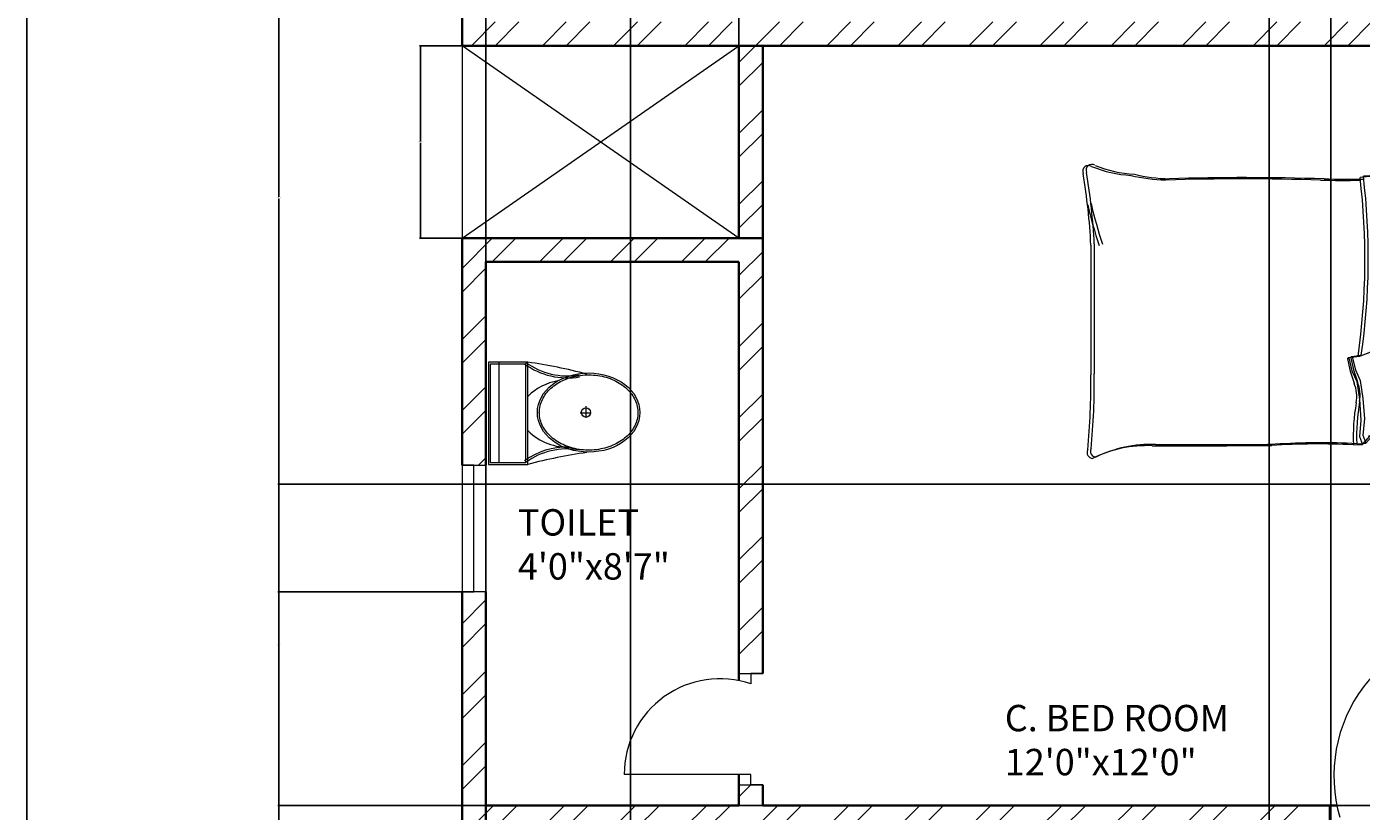
# Model space of a CAD drawing. Units: inches. Extents: x 1965 to 2673, y 1802 to 2669.
# Tile 7 of 16: x 1965 to 2218, y 2267 to 2416. Entities that reach past the tile are written whole.
import ezdxf

# ---------------------------------------------------------------- set-up
doc = ezdxf.new("R2010")
doc.units = ezdxf.units.IN
for name, color, linetype, lineweight in [('A-ANNO-DIMS', 2, 'Continuous', 18), ('A-ANNO-TTLB', 7, 'Continuous', 25), ('A-AREA-IDEN', 7, 'Continuous', 18), ('A-DOOR', 11, 'Continuous', 18), ('A-FLOR-FIXT', 9, 'Continuous', 18), ('A-FLOR-OPEN', 8, 'Continuous', 13), ('A-FURN', 8, 'Continuous', 13), ('A-GLAZ', 181, 'Continuous', 18), ('A-WALL', 7, 'Continuous', 35), ('A-WALL-PATT', 252, 'Continuous', 13)]:
    doc.layers.add(name, color=color, linetype=linetype, lineweight=lineweight)
doc.styles.get("Standard").update_dxf_attribs({"font": 'arial.ttf'})
doc.dimstyles.get("Standard").update_dxf_attribs({"dimtxt": 0.18, "dimasz": 0.18, "dimexe": 0.18, "dimexo": 0.0625, "dimgap": 0.09, "dimtad": 0, "dimtih": 1, "dimtoh": 1, "dimdec": 4, "dimzin": 0, "dimdsep": 46, "dimtxsty": 'Standard', "dimcen": 0.09, "dimadec": 0, "dimazin": 0, "dimtfac": 1, "dimtdec": 4, "dimtofl": 0, "dimtmove": 0, "dimatfit": 3, "dimfxl": 1, "dimtolj": 1, "dimtzin": 0, "dimarcsym": 0})

# ---------------------------------------------------------------- blocks, each defined once
blk = doc.blocks.new('A$C31115884')
for p, q in [((283.1, 497.7), (223.4, 497.7)), ((257.5, 466.4), (257.5, 523.2)), ((0, 200), (0, 0)), ((520, 200), (0, 200)), ((10, 190), (10, 10)), ((510, 190), (10, 190)), ((510, 10), (510, 190)), ((520, 0), (520, 200)), ((510, 54.5), (0, 54.5)), ((10, 10), (510, 10)), ((0, 0), (520, 0))]:
    blk.add_line(p, q)
blk.add_circle((255.6, 496.4), 23.6)
for centre, radius, start, end in [((2777.7, -204.6), 2807, 165.4549, 171.71327), ((3237, 905), 2807, 188.28673, 194.5451), ((-294.5, 403.3), 364.7, 324.20913, 9.34987), ((-294.5, 403.3), 374.7, 324.20913, 9.34987), ((139.5, 406.2), 293.5, 315.84364, 2.65635), ((805.8, 403.3), 374.7, 179.20365, 215.79087), ((805.8, 403.3), 364.7, 170.65013, 215.79087), ((383.6, 406.2), 293.5, 190.27735, 224.15636)]:
    blk.add_arc(centre, radius, start, end)
blk.add_ellipse((256.2, 509.9), major_axis=(0, -260.7), ratio=0.772727)
blk.add_open_spline([(256.2, 259.2), (263.1, 259.2), (270, 259.7), (287.8, 262.3), (298.7, 265.1), (319.9, 273.1), (330.2, 278.4), (350.1, 291.1), (359.7, 298.7), (377.7, 315.9), (386.2, 325.5), (401.7, 346.6), (408.8, 358.1), (421.3, 382.5), (426.8, 395.5), (435.9, 422.4), (439.5, 436.4), (444.8, 465.1), (446.5, 479.7), (447.9, 509.2), (447.6, 524), (445, 553.3), (442.7, 567.8), (436.3, 596), (432.1, 609.7), (421.9, 636), (416, 648.6), (402.5, 672.1), (395, 683), (378.6, 703), (369.8, 712.1), (351.1, 728), (341.3, 734.8), (320.9, 746.2), (310.4, 750.7), (288.9, 757.3), (278, 759.4), (256, 761), (245, 760.6), (223.1, 757.2), (212.3, 754.3), (191.1, 746.1), (180.8, 740.7), (160.9, 727.8), (151.4, 720.1), (133.5, 702.7), (125.1, 693), (109.6, 671.7), (102.6, 660.2), (90.2, 635.7), (84.9, 622.7), (76, 595.6), (72.4, 581.6), (67.2, 552.9), (65.6, 538.2), (64.4, 508.8), (64.8, 494), (67.5, 464.7), (69.9, 450.2), (76.6, 422), (80.8, 408.3), (91.1, 382.2), (97.2, 369.7), (110.8, 346.3), (118.4, 335.4), (134.8, 315.6), (143.7, 306.7), (162.4, 290.9), (172.3, 284.2), (192.8, 273), (203.3, 268.6), (224.8, 262.2), (235.8, 260.2), (249.9, 259.3), (253, 259.2), (256.2, 259.2)], degree=3, knots=[0, 0, 0, 0, 0.110105, 0.110105, 0.285049, 0.285049, 0.459994, 0.459994, 0.634938, 0.634938, 0.809882, 0.809882, 0.984827, 0.984827, 1.159771, 1.159771, 1.334715, 1.334715, 1.50966, 1.50966, 1.684604, 1.684604, 1.859549, 1.859549, 2.034493, 2.034493, 2.209437, 2.209437, 2.384382, 2.384382, 2.559326, 2.559326, 2.73427, 2.73427, 2.909215, 2.909215, 3.084159, 3.084159, 3.259103, 3.259103, 3.434048, 3.434048, 3.608992, 3.608992, 3.783936, 3.783936, 3.958881, 3.958881, 4.133825, 4.133825, 4.30877, 4.30877, 4.483714, 4.483714, 4.658658, 4.658658, 4.833603, 4.833603, 5.008547, 5.008547, 5.183491, 5.183491, 5.358436, 5.358436, 5.53338, 5.53338, 5.708324, 5.708324, 5.883269, 5.883269, 6.058213, 6.058213, 6.233158, 6.233158, 6.283185, 6.283185, 6.283185, 6.283185])
blk = doc.blocks.new('BED-DOUBLE')
for p, q in [((3.47, 63.33), (3.47, 81.44)), ((3.47, 63.33), (3.47, 81.44)), ((3.47, 81.44), (51.49, 81.44)), ((51.26, 81.44), (51.26, 54.83)), ((51.26, 81.44), (51.26, 54.83)), ((51.49, 81.44), (51.49, 80.8)), ((3.47, 79.91), (51.26, 79.91)), ((3.47, 79.91), (51.26, 79.91)), ((3.7, 62.69), (3.7, 80.8)), ((3.7, 62.69), (3.7, 80.8)), ((3.7, 79.27), (51.49, 79.27)), ((3.7, 79.27), (51.49, 79.27)), ((3.89, 78.1), (8.17, 78.43)), ((3.89, 78.1), (8.17, 78.43)), ((8.17, 78.43), (8.28, 78.41)), ((8.17, 78.43), (8.28, 78.41)), ((16.87, 78.41), (19.76, 79.14)), ((16.87, 78.41), (19.76, 79.14)), ((17.1, 77.77), (19.99, 78.5)), ((17.1, 77.77), (19.99, 78.5)), ((19.76, 79.14), (20.09, 79.14)), ((19.76, 79.14), (20.09, 79.14)), ((19.99, 78.5), (20.31, 78.5)), ((19.99, 78.5), (20.31, 78.5)), ((20.09, 79.14), (24.53, 78.99)), ((20.09, 79.14), (24.53, 78.99)), ((20.31, 78.5), (24.76, 78.35)), ((20.31, 78.5), (24.76, 78.35)), ((24.53, 78.99), (25.98, 79.57)), ((24.53, 78.99), (25.98, 79.57)), ((24.76, 78.35), (26.21, 78.93)), ((24.76, 78.35), (26.21, 78.93)), ((25.98, 79.57), (26.56, 74.22)), ((25.98, 79.57), (26.56, 74.22)), ((26.21, 78.93), (26.78, 73.58)), ((26.21, 78.93), (26.78, 73.58)), ((27.97, 78.95), (27.73, 73.57)), ((27.97, 78.95), (27.73, 73.57)), ((29.45, 78.46), (27.97, 78.95)), ((29.45, 78.46), (27.97, 78.95)), ((33.88, 78.88), (29.45, 78.46)), ((33.88, 78.88), (29.45, 78.46)), ((34.2, 78.9), (33.88, 78.88)), ((34.2, 78.9), (33.88, 78.88)), ((37.13, 78.36), (34.2, 78.9)), ((37.13, 78.36), (34.2, 78.9)), ((45.71, 78.9), (41.91, 78.37)), ((45.71, 78.9), (41.91, 78.37)), ((50.11, 78.88), (44.7, 78.98)), ((44.7, 78.98), (45.71, 78.9)), ((50.11, 78.88), (44.7, 78.98)), ((44.7, 78.98), (45.71, 78.9)), ((50.11, 78.88), (49.73, 75.67)), ((50.11, 78.88), (49.73, 75.67)), ((51.49, 80.8), (51.49, 54.19)), ((51.49, 80.8), (51.49, 54.19)), ((3.89, 78.12), (4.47, 74.94)), ((3.89, 78.12), (4.47, 74.94)), ((4.12, 77.46), (8.4, 77.79)), ((4.12, 77.46), (8.4, 77.79)), ((4.12, 77.49), (4.7, 74.3)), ((4.12, 77.49), (4.7, 74.3)), ((8.28, 78.41), (12.1, 78.12)), ((8.28, 78.41), (12.1, 78.12)), ((8.4, 77.79), (8.51, 77.77)), ((8.4, 77.79), (8.51, 77.77)), ((8.51, 77.77), (12.33, 77.49)), ((8.51, 77.77), (12.33, 77.49)), ((12.1, 78.12), (17.6, 77.11)), ((12.1, 78.12), (17.6, 77.11)), ((12.33, 77.49), (17.82, 76.47)), ((12.33, 77.49), (17.82, 76.47)), ((14.85, 77.69), (16.87, 78.41)), ((14.85, 77.69), (16.87, 78.41)), ((15.08, 77.05), (17.1, 77.77)), ((15.08, 77.05), (17.1, 77.77)), ((28.2, 78.31), (27.96, 72.93)), ((28.2, 78.31), (27.96, 72.93)), ((29.68, 77.82), (28.2, 78.31)), ((29.68, 77.82), (28.2, 78.31)), ((34.11, 78.24), (29.68, 77.82)), ((34.11, 78.24), (29.68, 77.82)), ((34.43, 78.26), (34.11, 78.24)), ((34.43, 78.26), (34.11, 78.24)), ((37.36, 77.72), (34.43, 78.26)), ((37.36, 77.72), (34.43, 78.26)), ((41.91, 78.37), (36.49, 77.02)), ((41.91, 78.37), (36.49, 77.02)), ((42.14, 77.73), (36.72, 76.38)), ((42.14, 77.73), (36.72, 76.38)), ((39.2, 77.77), (37.13, 78.36)), ((39.19, 77.77), (37.13, 78.36)), ((39.42, 77.13), (37.36, 77.72)), ((39.42, 77.13), (37.36, 77.72)), ((45.94, 78.26), (42.14, 77.73)), ((45.94, 78.26), (42.14, 77.73)), ((50.34, 78.24), (44.93, 78.34)), ((44.93, 78.34), (45.94, 78.26)), ((50.34, 78.24), (44.93, 78.34)), ((44.93, 78.34), (45.94, 78.26)), ((50.34, 78.24), (49.96, 75.03)), ((50.34, 78.24), (49.96, 75.03)), ((4.47, 74.94), (4.03, 72.34)), ((4.47, 74.94), (4.03, 72.34)), ((4.7, 74.3), (4.26, 71.7)), ((4.7, 74.3), (4.26, 71.7)), ((5.05, 72.49), (6.06, 75.23)), ((5.05, 72.49), (6.06, 75.23)), ((5.27, 71.85), (6.29, 74.59)), ((5.27, 71.85), (6.29, 74.59)), ((26.56, 74.22), (27.13, 71.04)), ((26.56, 74.22), (27.13, 71.04)), ((26.78, 73.58), (27.36, 70.4)), ((26.78, 73.58), (27.36, 70.4)), ((27.73, 73.57), (27.35, 70.36)), ((27.73, 73.57), (27.35, 70.36)), ((49.3, 73.18), (48.12, 75.86)), ((49.3, 73.18), (48.12, 75.86)), ((49.53, 72.54), (48.35, 75.22)), ((49.53, 72.54), (48.35, 75.22)), ((49.73, 75.67), (50.32, 73.1)), ((49.73, 75.67), (50.32, 73.1)), ((49.96, 75.03), (50.55, 72.46)), ((49.96, 75.03), (50.55, 72.46)), ((4.03, 72.34), (4.61, 71.33)), ((4.03, 72.34), (4.61, 71.33)), ((4.26, 71.7), (4.84, 70.69)), ((4.26, 71.7), (4.84, 70.69)), ((4.47, 68.87), (5.05, 72.49)), ((4.47, 68.87), (5.05, 72.49)), ((4.7, 68.23), (5.27, 71.85)), ((4.7, 68.23), (5.27, 71.85)), ((27.13, 71.04), (27.13, 69.74)), ((27.13, 71.04), (27.13, 69.74)), ((27.96, 72.93), (27.58, 69.72)), ((27.96, 72.93), (27.58, 69.72)), ((50.11, 69.61), (49.3, 73.18)), ((50.11, 69.61), (49.3, 73.18)), ((50.34, 68.97), (49.53, 72.54)), ((50.34, 68.97), (49.53, 72.54)), ((50.32, 73.1), (49.81, 72.06)), ((50.32, 73.1), (49.81, 72.06)), ((50.55, 72.46), (50.04, 71.42)), ((50.55, 72.46), (50.04, 71.42)), ((4.76, 67.28), (4.47, 68.87)), ((4.76, 67.28), (4.47, 68.87)), ((27.13, 69.74), (26.56, 67.86)), ((27.13, 69.74), (26.56, 67.86)), ((27.36, 69.1), (26.78, 67.22)), ((27.36, 69.1), (26.78, 67.22)), ((27.35, 70.36), (27.43, 69.06)), ((27.35, 70.36), (27.43, 69.06)), ((27.36, 70.4), (27.36, 69.1)), ((27.36, 70.4), (27.36, 69.1)), ((27.43, 69.06), (28.13, 67.22)), ((27.43, 69.06), (28.13, 67.22)), ((27.58, 69.72), (27.66, 68.42)), ((27.58, 69.72), (27.66, 68.42)), ((27.66, 68.42), (28.35, 66.58)), ((27.66, 68.42), (28.35, 66.58)), ((49.92, 68.01), (50.11, 69.61)), ((49.92, 68.01), (50.11, 69.61)), ((50.15, 67.37), (50.34, 68.97)), ((50.15, 67.37), (50.34, 68.97)), ((4.18, 64.1), (4.76, 67.28)), ((4.18, 64.1), (4.76, 67.28)), ((4.41, 63.46), (4.99, 66.64)), ((4.41, 63.46), (4.99, 66.64)), ((4.99, 66.64), (4.7, 68.23)), ((4.99, 66.64), (4.7, 68.23)), ((6.38, 65.81), (10.41, 65.15)), ((6.38, 65.81), (10.41, 65.15)), ((24.1, 65.18), (20.95, 66.27)), ((24.1, 65.18), (20.95, 66.27)), ((26.56, 67.86), (26.56, 65.18)), ((26.56, 67.86), (26.56, 65.18)), ((26.78, 67.22), (26.78, 64.54)), ((26.78, 67.22), (26.78, 64.54)), ((28.13, 67.22), (28.29, 64.55)), ((28.13, 67.22), (28.29, 64.55)), ((28.35, 66.58), (28.52, 63.91)), ((28.35, 66.58), (28.52, 63.91)), ((30.75, 64.7), (33.82, 65.99)), ((30.75, 64.7), (33.82, 65.99)), ((32.56, 65.81), (36.59, 65.15)), ((32.56, 65.81), (36.59, 65.15)), ((50.69, 64.87), (49.92, 68.01)), ((50.69, 64.87), (49.92, 68.01)), ((50.92, 64.23), (50.15, 67.37)), ((50.92, 64.23), (50.15, 67.37)), ((9.28, 64.82), (4.18, 64.1)), ((9.28, 64.82), (4.18, 64.1)), ((9.5, 64.18), (4.41, 63.46)), ((9.5, 64.18), (4.41, 63.46)), ((6.6, 65.17), (10.64, 64.51)), ((6.61, 65.17), (10.64, 64.51)), ((10.41, 65.15), (9.28, 64.82)), ((10.41, 65.15), (9.28, 64.82)), ((10.64, 64.51), (9.5, 64.18)), ((10.64, 64.51), (9.5, 64.18)), ((10.41, 65.15), (17.42, 64.71)), ((10.41, 65.15), (17.42, 64.71)), ((10.64, 64.51), (17.65, 64.08)), ((10.64, 64.51), (17.65, 64.08)), ((17.42, 64.71), (19.38, 65.27)), ((17.42, 64.71), (19.38, 65.27)), ((17.65, 64.08), (19.61, 64.63)), ((17.65, 64.08), (19.61, 64.63)), ((19.38, 65.27), (24.51, 64.87)), ((19.38, 65.27), (24.51, 64.87)), ((19.61, 64.63), (24.74, 64.23)), ((19.61, 64.63), (24.74, 64.23)), ((24.33, 64.54), (21.18, 65.63)), ((24.33, 64.54), (21.18, 65.63)), ((26.56, 65.18), (24.1, 65.18)), ((26.56, 65.18), (24.1, 65.18)), ((26.78, 64.54), (24.33, 64.54)), ((26.78, 64.54), (24.33, 64.54)), ((28.29, 64.55), (30.75, 64.7)), ((28.29, 64.55), (30.75, 64.7)), ((28.52, 63.91), (30.97, 64.06)), ((28.52, 63.91), (30.97, 64.06)), ((30.25, 64.06), (34.44, 57.56)), ((30.25, 64.06), (34.44, 57.56)), ((30.48, 63.42), (34.67, 56.92)), ((30.48, 63.42), (34.67, 56.92)), ((30.97, 64.06), (34.04, 65.35)), ((30.97, 64.06), (34.04, 65.35)), ((40.64, 61.12), (32.3, 64.06)), ((40.64, 61.12), (32.3, 64.06)), ((40.87, 60.48), (32.53, 63.42)), ((40.87, 60.48), (32.53, 63.42)), ((32.79, 65.17), (36.82, 64.51)), ((32.79, 65.17), (36.82, 64.51)), ((36.59, 65.15), (43.6, 64.71)), ((36.59, 65.15), (43.6, 64.71)), ((36.82, 64.51), (43.83, 64.08)), ((36.82, 64.51), (43.83, 64.08)), ((43.6, 64.71), (45.56, 65.27)), ((43.6, 64.71), (45.56, 65.27)), ((43.83, 64.08), (45.79, 64.63)), ((43.83, 64.08), (45.79, 64.63)), ((45.56, 65.27), (50.69, 64.87)), ((45.56, 65.27), (50.69, 64.87)), ((45.79, 64.63), (50.92, 64.23)), ((45.79, 64.63), (50.92, 64.23)), ((46.21, 59.11), (40.64, 61.12)), ((46.21, 59.11), (40.64, 61.12)), ((46.44, 58.47), (40.87, 60.48)), ((46.44, 58.47), (40.87, 60.48)), ((49.16, 56.95), (46.21, 59.11)), ((49.16, 56.95), (46.21, 59.11)), ((49.39, 56.31), (46.44, 58.47)), ((49.39, 56.31), (46.44, 58.47)), ((34.44, 57.56), (36.15, 53.08)), ((34.44, 57.56), (36.15, 53.08)), ((34.67, 56.92), (36.38, 52.44)), ((34.67, 56.92), (36.38, 52.44)), ((52.86, 53.69), (49.16, 56.95)), ((52.86, 53.69), (49.16, 56.95)), ((53.09, 53.06), (49.39, 56.31)), ((53.09, 53.06), (49.39, 56.31)), ((44.36, 53.08), (48.23, 53.39)), ((44.36, 53.08), (48.23, 53.39)), ((48.23, 53.39), (51.33, 53.08)), ((48.23, 53.39), (51.33, 53.08)), ((51.33, 53.08), (52.86, 53.69)), ((51.33, 53.08), (52.86, 53.69)), ((52.94, 51.95), (52.86, 53.69, 3.87)), ((52.94, 51.95), (52.86, 53.69, 3.87)), ((36.15, 53.08), (36.46, 51.06)), ((36.15, 53.08), (36.46, 51.06)), ((36.38, 52.44), (36.69, 50.42)), ((36.38, 52.44), (36.69, 50.42)), ((36.46, 51.06), (38.94, 51.68)), ((36.46, 51.06), (38.94, 51.68)), ((36.69, 50.42), (39.16, 51.04)), ((36.69, 50.42), (39.16, 51.04)), ((38.94, 51.68), (40.95, 52.61)), ((38.94, 51.68), (40.95, 52.61)), ((39.16, 51.04), (41.18, 51.97)), ((39.16, 51.04), (41.18, 51.97)), ((40.95, 52.61), (44.36, 53.08)), ((40.95, 52.61), (44.36, 53.08)), ((41.18, 51.97), (44.58, 52.44)), ((41.18, 51.97), (44.58, 52.44)), ((44.58, 52.44), (48.46, 52.75)), ((44.58, 52.44), (48.46, 52.75)), ((48.46, 52.75), (51.55, 52.44)), ((48.46, 52.75), (51.55, 52.44)), ((51.55, 52.44), (53.09, 53.06)), ((51.55, 52.44), (53.09, 53.06)), ((53.17, 51.31), (53.09, 53.06, 3.87)), ((53.17, 51.31), (53.09, 53.06, 3.87)), ((15.06, 2.2), (39.67, 2.2)), ((15.06, 2.2), (39.67, 2.2)), ((15.29, 1.56), (39.9, 1.56)), ((15.29, 1.56), (39.9, 1.56))]:
    blk.add_line(p, q)
for centre, radius, start, end in [((21.35, -100.61), 164.97, 86.0865, 96.7821), ((21.35, -100.61), 164.97, 86.0865, 96.7821), ((21.58, -101.25), 164.97, 86.0865, 96.7821), ((21.58, -101.25), 164.97, 86.0865, 96.7821), ((85.16, 61.34), 83.31, 178.7218, 185.604), ((85.16, 61.34), 83.31, 178.7218, 185.604), ((85.39, 60.71), 83.31, 178.7218, 185.604), ((85.38, 60.71), 83.31, 178.7218, 185.604), ((17.75, -74.88), 129.02, 81.7845, 96.9006), ((17.75, -74.88), 129.02, 81.7845, 96.9006), ((17.98, -75.51), 129.02, 81.7845, 96.9006), ((17.98, -75.51), 129.02, 81.7845, 96.9006), ((-167.31, 50.27), 170.11, 358.4762, 1.0082), ((-167.31, 50.27), 170.11, 358.4762, 1.0082), ((-167.08, 49.63), 170.11, 358.4762, 1.0082), ((-167.08, 49.63), 170.11, 358.4762, 1.0082), ((36.63, 51), 0.185, 160.2464, 271.1377), ((36.63, 51), 0.185, 160.2464, 271.1377), ((31.15, 79.96), 29.65, 280.6617, 289.8806), ((31.15, 79.96), 29.65, 280.6617, 289.8806), ((31.38, 79.32), 29.65, 280.6617, 289.8806), ((31.38, 79.32), 29.65, 280.6617, 289.8806), ((43.74, 46.37), 6.22, 78.6608, 113.7384), ((43.74, 46.37), 6.22, 78.6608, 113.7384), ((43.97, 45.74), 6.22, 78.6608, 113.7384), ((43.97, 45.74), 6.22, 78.6608, 113.7384), ((51.32, 88.1), 36.18, 259.8763, 272.5657), ((51.32, 88.1), 36.18, 259.8763, 272.5657), ((51.55, 87.46), 36.18, 259.8763, 272.5657), ((51.55, 87.46), 36.18, 259.8763, 272.5657), ((182.26, 45.13), 129.5, 176.9791, 183.8365), ((182.26, 45.13), 129.5, 176.9791, 183.8365), ((182.49, 44.49), 129.5, 176.9791, 183.8365), ((182.49, 44.49), 129.5, 176.9791, 183.8365), ((36.86, 50.36), 0.185, 160.2464, 271.1377), ((36.86, 50.36), 0.185, 160.2464, 271.1377), ((484.82, 30.83), 482.31, 178.2277, 181.7185), ((484.82, 30.83), 482.31, 178.2277, 181.7185), ((485.05, 30.19), 482.31, 178.2277, 181.7185), ((485.05, 30.19), 482.31, 178.2277, 181.7185), ((-4508.75, 13.62), 4561.86, 0.00217, 0.28689), ((-4508.75, 13.62), 4561.86, 0.00217, 0.28689), ((-4508.52, 12.98), 4561.86, 0.00217, 0.28689), ((-4508.52, 12.98), 4561.86, 0.00217, 0.28689), ((-26.9, 16.93), 29.63, 346.0648, 358.9113), ((-26.9, 16.93), 29.63, 346.0648, 358.9113), ((-26.68, 16.29), 29.63, 346.0648, 358.9113), ((-26.68, 16.29), 29.63, 346.0648, 358.9113), ((76.15, 12.77), 23.07, 177.4714, 206.4681), ((76.15, 12.77), 23.07, 177.4714, 206.4681), ((76.38, 12.14), 23.07, 177.4714, 206.4681), ((76.38, 12.14), 23.07, 177.4714, 206.4681), ((-21.66, 11.17), 23.56, 337.9751, 356.652), ((-21.66, 11.17), 23.56, 337.9751, 356.652), ((-21.44, 10.53), 23.56, 337.9751, 356.652), ((-21.44, 10.53), 23.56, 337.9751, 356.652), ((-17.23, 105.15), 106.46, 283.3832, 287.7053), ((-17.23, 105.15), 106.46, 283.3832, 287.7053), ((-17, 104.51), 106.46, 283.3832, 287.7053), ((-17, 104.51), 106.46, 283.3832, 287.7053), ((1.08, 1.72), 1.09, 146.1736, 293.4781), ((1.08, 1.72), 1.09, 146.1736, 293.4781), ((1.31, 1.08), 1.09, 146.1736, 293.4781), ((1.31, 1.08), 1.09, 146.1736, 293.4781), ((21.42, -119.4), 121.76, 92.9958, 99.4091), ((21.42, -119.4), 121.76, 92.9958, 99.4091), ((21.65, -120.04), 121.76, 92.9958, 99.4091), ((21.65, -120.04), 121.76, 92.9958, 99.4091), ((41.15, -130.84), 133.04, 84.4998, 90.6351), ((41.15, -130.84), 133.04, 84.4998, 90.6351), ((41.38, -131.48), 133.04, 84.4998, 90.6351), ((41.37, -131.48), 133.04, 84.4998, 90.6351), ((54.4, 2.57), 1.1, 242.6588, 356.02), ((54.4, 2.57), 1.1, 242.6588, 356.02), ((54.63, 1.93), 1.1, 242.6588, 356.02), ((54.63, 1.93), 1.1, 242.6588, 356.02)]:
    blk.add_arc(centre, radius, start, end)
blk = doc.blocks.new('SHAFT-OPENING')
for p, q in [((0, 36.5), (0, 0)), ((52.5, 0), (0, 36.5)), ((0, 0), (52.5, 36.5))]:
    blk.add_line(p, q)
blk = doc.blocks.new('*D23')
at = {"layer": 'A-ANNO-DIMS', "color": 0, "lineweight": -2, "transparency": 16777216}
for p, q in [((2047.09, 2412.65), (2047.09, 2420.65)), ((2047.27, 2420.47), (2072.37, 2420.47)), ((2099.41, 2420.47), (2074.32, 2420.47)), ((2099.59, 2412.65), (2099.59, 2420.65))]:
    blk.add_line(p, q, dxfattribs=at)
at = {"layer": 'A-ANNO-DIMS', "color": 0, "transparency": 16777216}
for points in [[(2047.27, 2420.5), (2047.27, 2420.44), (2047.09, 2420.47)], [(2099.41, 2420.5), (2099.41, 2420.44), (2099.59, 2420.47)]]:
    blk.add_solid(points, dxfattribs=at)
at = {"layer": 'Defpoints', "color": 0, "transparency": 16777216}
for p in [(2099.59, 2420.47), (2047.09, 2412.59), (2099.59, 2412.59)]:
    blk.add_point(p, dxfattribs=at)
at = {"layer": 'A-ANNO-DIMS', "color": 0, "transparency": 16777216, "insert": (2073.34, 2420.47), "char_height": 0.18, "attachment_point": 5}
blk.add_mtext('\\A1;SHAFT 53 TYP.', dxfattribs=at)
blk = doc.blocks.new('*D24')
at = {"layer": 'A-ANNO-DIMS', "color": 0, "lineweight": -2, "transparency": 16777216}
for p, q in [((2047.03, 2412.59), (2039.04, 2412.59)), ((2039.22, 2412.41), (2039.22, 2394.52)), ((2039.22, 2376.27), (2039.22, 2394.16)), ((2047.03, 2376.09), (2039.04, 2376.09))]:
    blk.add_line(p, q, dxfattribs=at)
at = {"layer": 'A-ANNO-DIMS', "color": 0, "transparency": 16777216}
for points in [[(2039.19, 2412.41), (2039.25, 2412.41), (2039.22, 2412.59)], [(2039.19, 2376.27), (2039.25, 2376.27), (2039.22, 2376.09)]]:
    blk.add_solid(points, dxfattribs=at)
at = {"layer": 'Defpoints', "color": 0, "transparency": 16777216}
for p in [(2039.22, 2412.59), (2047.09, 2412.59), (2047.09, 2376.09)]:
    blk.add_point(p, dxfattribs=at)
at = {"layer": 'A-ANNO-DIMS', "color": 0, "transparency": 16777216, "insert": (2039.22, 2394.34), "char_height": 0.18, "attachment_point": 5}
blk.add_mtext('\\A1;37 TYP.', dxfattribs=at)
blk = doc.blocks.new('*D36')
at = {"layer": 'A-ANNO-DIMS', "color": 0, "lineweight": -2, "transparency": 16777216}
for p, q in [((2047.03, 2309.07), (2012.19, 2309.07)), ((2012.37, 2308.89), (2012.37, 2253.51)), ((2012.37, 2197.76), (2012.37, 2253.14)), ((2047.03, 2197.58), (2012.19, 2197.58))]:
    blk.add_line(p, q, dxfattribs=at)
at = {"layer": 'A-ANNO-DIMS', "color": 0, "transparency": 16777216}
for points in [[(2012.34, 2308.89), (2012.4, 2308.89), (2012.37, 2309.07)], [(2012.34, 2197.76), (2012.4, 2197.76), (2012.37, 2197.58)]]:
    blk.add_solid(points, dxfattribs=at)
at = {"layer": 'Defpoints', "color": 0, "transparency": 16777216}
for p in [(2012.37, 2309.07), (2047.09, 2309.07), (2047.09, 2197.58)]:
    blk.add_point(p, dxfattribs=at)
at = {"layer": 'A-ANNO-DIMS', "color": 0, "transparency": 16777216, "insert": (2012.37, 2253.33), "char_height": 0.18, "attachment_point": 5}
blk.add_mtext('\\A1;111.49', dxfattribs=at)
blk = doc.blocks.new('*D37')
at = {"layer": 'A-ANNO-DIMS', "color": 0, "lineweight": -2, "transparency": 16777216}
for p, q in [((2047.03, 2458.38), (2012.19, 2458.38)), ((2012.37, 2458.2), (2012.37, 2383.91)), ((2012.37, 2309.25), (2012.37, 2383.54)), ((2047.03, 2309.07), (2012.19, 2309.07))]:
    blk.add_line(p, q, dxfattribs=at)
at = {"layer": 'A-ANNO-DIMS', "color": 0, "transparency": 16777216}
for points in [[(2012.34, 2458.2), (2012.4, 2458.2), (2012.37, 2458.38)], [(2012.34, 2309.25), (2012.4, 2309.25), (2012.37, 2309.07)]]:
    blk.add_solid(points, dxfattribs=at)
at = {"layer": 'Defpoints', "color": 0, "transparency": 16777216}
for p in [(2012.37, 2458.38), (2047.09, 2458.38), (2047.09, 2309.07)]:
    blk.add_point(p, dxfattribs=at)
at = {"layer": 'A-ANNO-DIMS', "color": 0, "transparency": 16777216, "insert": (2012.37, 2383.73), "char_height": 0.18, "attachment_point": 5}
blk.add_mtext('\\A1;149.3', dxfattribs=at)
blk = doc.blocks.new('*D39')
at = {"layer": 'A-ANNO-DIMS', "color": 0, "lineweight": -2, "transparency": 16777216}
for p, q in [((2051.59, 1936.15), (2051.59, 2600.5)), ((2051.77, 2600.32), (2064.93, 2600.32)), ((2078.87, 2600.32), (2065.72, 2600.32)), ((2079.05, 1936.15), (2079.05, 2600.5))]:
    blk.add_line(p, q, dxfattribs=at)
at = {"layer": 'A-ANNO-DIMS', "color": 0, "transparency": 16777216}
for points in [[(2051.77, 2600.35), (2051.77, 2600.29), (2051.59, 2600.32)], [(2078.87, 2600.35), (2078.87, 2600.29), (2079.05, 2600.32)]]:
    blk.add_solid(points, dxfattribs=at)
at = {"layer": 'Defpoints', "color": 0, "transparency": 16777216}
for p in [(2079.05, 2600.32), (2051.59, 1936.09), (2079.05, 1936.09)]:
    blk.add_point(p, dxfattribs=at)
at = {"layer": 'A-ANNO-DIMS', "color": 0, "transparency": 16777216, "insert": (2065.32, 2600.32), "char_height": 0.18, "attachment_point": 5}
blk.add_mtext('\\A1;27.46', dxfattribs=at)
blk = doc.blocks.new('*D40')
at = {"layer": 'A-ANNO-DIMS', "color": 0, "lineweight": -2, "transparency": 16777216}
for p, q in [((2200.09, 1936.15), (2200.09, 2600.5)), ((2200.27, 2600.32), (2205.48, 2600.32)), ((2211.59, 2600.32), (2206.38, 2600.32)), ((2211.77, 1936.15), (2211.77, 2600.5))]:
    blk.add_line(p, q, dxfattribs=at)
at = {"layer": 'A-ANNO-DIMS', "color": 0, "transparency": 16777216}
for points in [[(2200.27, 2600.35), (2200.27, 2600.29), (2200.09, 2600.32)], [(2211.59, 2600.35), (2211.59, 2600.29), (2211.77, 2600.32)]]:
    blk.add_solid(points, dxfattribs=at)
at = {"layer": 'Defpoints', "color": 0, "transparency": 16777216}
for p in [(2211.77, 2600.32), (2200.09, 1936.09), (2211.77, 1936.09)]:
    blk.add_point(p, dxfattribs=at)
at = {"layer": 'A-ANNO-DIMS', "color": 0, "transparency": 16777216, "insert": (2205.93, 2600.32), "char_height": 0.18, "attachment_point": 5}
blk.add_mtext('\\A1;11.674', dxfattribs=at)
blk = doc.blocks.new('*D48')
at = {"layer": 'A-ANNO-DIMS', "color": 0, "lineweight": -2, "transparency": 16777216}
for p, q in [((2573.53, 2329.47), (2012.19, 2329.47)), ((2012.37, 2329.29), (2012.37, 2299.21)), ((2012.37, 2268.77), (2012.37, 2298.85)), ((2573.53, 2268.59), (2012.19, 2268.59))]:
    blk.add_line(p, q, dxfattribs=at)
at = {"layer": 'A-ANNO-DIMS', "color": 0, "transparency": 16777216}
for points in [[(2012.34, 2329.29), (2012.4, 2329.29), (2012.37, 2329.47)], [(2012.34, 2268.77), (2012.4, 2268.77), (2012.37, 2268.59)]]:
    blk.add_solid(points, dxfattribs=at)
at = {"layer": 'Defpoints', "color": 0, "transparency": 16777216}
for p in [(2012.37, 2329.47), (2573.59, 2329.47), (2573.59, 2268.59)]:
    blk.add_point(p, dxfattribs=at)
at = {"layer": 'A-ANNO-DIMS', "color": 0, "transparency": 16777216, "insert": (2012.37, 2299.03), "char_height": 0.18, "attachment_point": 5}
blk.add_mtext('\\A1;60.87', dxfattribs=at)

msp = doc.modelspace()

# ---------------------------------------------------------------- hatches: boundary and pattern name
at = {"layer": 'A-WALL-PATT'}
h = msp.add_hatch(dxfattribs=at)
h.set_pattern_fill('ANSI32', color=256)
h.paths.add_polyline_path([(2051.5927, 2561.0914), (2076.7559, 2561.0914), (2076.7559, 2563.3414), (2076.7559, 2565.5914), (2047.0927, 2565.5914), (2047.0927, 2518.3824), (2051.5927, 2518.3824)])
h.paths.add_polyline_path([(2051.5927, 2458.3824), (2049.3427, 2458.3824), (2047.0927, 2458.3824), (2047.0927, 2412.5914), (2248.0927, 2412.5914), (2248.0927, 2268.5914), (2252.5927, 2268.5914), (2252.5927, 2412.5914), (2252.5927, 2421.0404), (2250.3427, 2421.0404), (2248.0927, 2421.0404), (2248.0927, 2417.0914), (2051.5927, 2417.0914)])
h.paths.add_polyline_path([(2211.4933, 2268.5914), (2104.0927, 2268.5914), (2104.0927, 2272.4654), (2101.8427, 2272.4654), (2099.5927, 2272.4654), (2099.5927, 2268.5914), (2051.5927, 2268.5914), (2051.5927, 2264.0914), (2147.5927, 2264.0914), (2147.5927, 2259.8893), (2152.0927, 2259.8893), (2152.0927, 2264.0914), (2211.4933, 2264.0914), (2211.4933, 2266.3414)])
h.paths.add_polyline_path([(2104.0927, 2376.0914), (2099.5927, 2376.0914), (2047.0927, 2376.0914), (2047.0927, 2333.0682), (2051.5927, 2333.0682), (2051.5927, 2371.5914), (2099.5927, 2371.5914), (2099.5927, 2293.6123), (2104.0927, 2293.6123)], flags=17)
h.paths.add_polyline_path([(2051.5927, 2309.0682), (2047.0927, 2309.0682), (2047.0927, 2233.5821), (2051.5927, 2233.5821)])
h.paths.add_polyline_path([(2104.0927, 2412.5914), (2099.5927, 2412.5914), (2099.5927, 2376.0914), (2104.0927, 2376.0914)], flags=17)
h.paths.add_polyline_path([(2290.1254, 2268.5914), (2242.4924, 2268.5914), (2242.4924, 2264.0914), (2290.1254, 2264.0914), (2290.1254, 2266.3414)])
h.paths.add_polyline_path([(2284.653, 2264.0914), (2280.153, 2264.0914), (2280.153, 2161.6826), (2284.653, 2161.6826)])
h.paths.add_polyline_path([(2578.0927, 2329.4656), (2573.5927, 2329.4656), (2573.5927, 2268.5914), (2525.5927, 2268.5914), (2525.5927, 2271.9222), (2523.3427, 2271.9222), (2521.0927, 2271.9222), (2521.0927, 2268.5914), (2324.2835, 2268.5914), (2324.2835, 2264.0914), (2329.0927, 2264.0914), (2329.0927, 2259.4977), (2333.5927, 2259.4977), (2333.5927, 2264.0914), (2473.0927, 2264.0914), (2473.0927, 2259.9371), (2477.5927, 2259.9371), (2477.5927, 2264.0914), (2573.5927, 2264.0914), (2573.5927, 2235.5751), (2578.0927, 2235.5751)])
h.paths.add_polyline_path([(2377.0927, 2412.5914), (2578.0927, 2412.5914), (2578.0927, 2444.2286), (2575.8427, 2444.2286), (2573.5927, 2444.2286), (2573.5927, 2417.0914), (2429.5927, 2417.0914), (2377.0927, 2417.0914), (2377.0927, 2421.7443), (2372.5927, 2421.7443), (2372.5927, 2268.5914), (2377.0927, 2268.5914)])
h.paths.add_polyline_path([(2525.5927, 2371.5914), (2573.5927, 2371.5914), (2573.5927, 2353.4656), (2578.0927, 2353.4656), (2578.0927, 2376.0914), (2525.5927, 2376.0914), (2521.0927, 2376.0914), (2521.0927, 2290.6472), (2525.5927, 2290.6472)], flags=17)
h.paths.add_polyline_path([(2477.5927, 2236.4106), (2475.3427, 2236.4106), (2473.0927, 2236.4106), (2473.0927, 2084.5914), (2465.3309, 2084.5914), (2465.3309, 2080.0914), (2481.6764, 2080.0914), (2481.6764, 2082.3414), (2481.6764, 2084.5914), (2477.5927, 2084.5914), (2477.5927, 2151.5914), (2573.5927, 2151.5914), (2573.5927, 2130.2907), (2578.0927, 2130.2907), (2578.0927, 2199.5751), (2575.8427, 2199.5751), (2573.5927, 2199.5751), (2573.5927, 2156.0914), (2477.5927, 2156.0914)])
h.paths.add_polyline_path([(2573.5927, 2084.5914), (2505.5513, 2084.5914), (2505.5513, 2080.0914), (2573.5927, 2080.0914)], flags=17)
h.paths.add_polyline_path([(2578.0927, 2106.2907), (2575.8427, 2106.2907), (2573.5927, 2106.2907), (2573.5927, 2050.8986), (2578.0927, 2050.8986)])
h.paths.add_polyline_path([(2578.0927, 1990.8986), (2575.8427, 1990.8986), (2573.5927, 1990.8986), (2573.5927, 1936.0914), (2522.132, 1936.0914), (2522.132, 1931.5914), (2578.0927, 1931.5914)])
h.paths.add_polyline_path([(2462.132, 1936.0914), (2429.5927, 1936.0914), (2429.5927, 2080.0914), (2432.623, 2080.0914), (2432.623, 2082.3414), (2432.623, 2084.5914), (2429.5927, 2084.5914), (2429.5927, 2120.5914), (2333.5927, 2120.5914), (2333.5927, 2229.3125), (2331.3427, 2229.3125), (2329.0927, 2229.3125), (2329.0927, 2116.0914), (2425.0927, 2116.0914), (2425.0927, 1936.0914), (2346.4058, 1936.0914), (2346.4058, 1931.5914), (2462.132, 1931.5914), (2462.132, 1933.8414)])
h.paths.add_polyline_path([(2211.767, 1933.8414), (2211.767, 1936.0914), (2200.0927, 1936.0914), (2200.0927, 2080.0914), (2200.0927, 2116.0914), (2284.653, 2116.0914), (2284.653, 2130.591), (2282.403, 2130.591), (2280.153, 2130.591), (2280.153, 2120.5914), (2200.0927, 2120.5914), (2195.5927, 2120.5914), (2195.5927, 2080.0914), (2195.5927, 1936.0914), (2139.0533, 1936.0914), (2139.0533, 1931.5914), (2211.767, 1931.5914)])
h.paths.add_polyline_path([(2282.2502, 1933.8414), (2282.2502, 1936.0914), (2259.767, 1936.0914), (2259.767, 1931.5914), (2282.2502, 1931.5914)], flags=17)
h.paths.add_polyline_path([(2051.5927, 1987.096), (2049.3427, 1987.096), (2047.0927, 1987.096), (2047.0927, 1931.5914), (2079.0533, 1931.5914), (2079.0533, 1933.8414), (2079.0533, 1936.0914), (2051.5927, 1936.0914)])
h.paths.add_polyline_path([(2051.5927, 2197.5821), (2049.3427, 2197.5821), (2047.0927, 2197.5821), (2047.0927, 2141.952), (2051.5927, 2141.952), (2051.5927, 2151.5914), (2147.5927, 2151.5914), (2147.5927, 2084.5914), (2144.3652, 2084.5914), (2144.3652, 2080.0914), (2155.9662, 2080.0914), (2155.9662, 2082.3414), (2155.9662, 2084.5914), (2152.0927, 2084.5914), (2152.0927, 2239.4921), (2149.8427, 2239.4921), (2147.5927, 2239.4921), (2147.5927, 2156.0914), (2051.5927, 2156.0914)])
h.paths.add_polyline_path([(2051.5927, 2080.0914), (2123.8575, 2080.0914), (2123.8575, 2082.3414), (2123.8575, 2084.5914), (2051.5927, 2084.5914), (2051.5927, 2117.952), (2047.0927, 2117.952), (2047.0927, 2047.096), (2051.5927, 2047.096)])
h = msp.add_hatch(dxfattribs=at)
h.set_pattern_fill('ANSI32', color=256)
h.paths.add_polyline_path([(2210.2316, 2563.3414), (2210.2316, 2565.5914), (2136.7559, 2565.5914), (2136.7559, 2561.0914), (2195.5927, 2561.0914), (2195.5927, 2485.8604), (2200.0927, 2485.8604), (2200.0927, 2561.0914), (2210.2316, 2561.0914)])
h.paths.add_polyline_path([(2285.9734, 2565.5914), (2234.2316, 2565.5914), (2234.2316, 2561.0914), (2248.0927, 2561.0914), (2248.0927, 2462.0914), (2200.0927, 2462.0914), (2200.0927, 2465.2357), (2197.8427, 2465.2357), (2195.5927, 2465.2357), (2195.5927, 2457.5914), (2248.0927, 2457.5914), (2248.0927, 2452.628), (2252.5927, 2452.628), (2252.5927, 2457.5914), (2257.5156, 2457.5914), (2257.5156, 2459.8414), (2257.5156, 2462.0914), (2252.5927, 2462.0914), (2252.5927, 2561.0914), (2285.9734, 2561.0914)])
h.paths.add_polyline_path([(2213.1374, 1872.8885), (2461.061, 1872.8885), (2461.061, 1909.9813), (2213.1374, 1909.9813)], flags=9)
h.paths.add_polyline_path([(2328.4056, 1942.3944), (2340.6089, 1942.3944), (2340.6089, 1952.6979), (2328.4056, 1952.6979)], flags=9)
h.paths.add_polyline_path([(2353.5759, 2030.9808), (2376.6455, 2030.9808), (2376.6455, 2041.2844), (2353.5759, 2041.2844)], flags=9)
h.paths.add_polyline_path([(2289.989, 2074.1041), (2326.916, 2074.1041), (2326.916, 2092.7615), (2289.989, 2092.7615)], flags=9)
h.paths.add_polyline_path([(2497.9, 2052.8638), (2548.3741, 2052.8638), (2548.3741, 2071.5212), (2497.9, 2071.5212)], flags=9)
h.paths.add_polyline_path([(2486.59, 2116.4883), (2515.7475, 2116.4883), (2515.7475, 2135.1456), (2486.59, 2135.1456)], flags=9)
h.paths.add_polyline_path([(2497.3007, 2181.2877), (2530.459, 2181.2877), (2530.459, 2199.945), (2497.3007, 2199.945)], flags=9)
h.paths.add_polyline_path([(2288.237, 2190.3228), (2324.1238, 2190.3228), (2324.1238, 2208.9802), (2288.237, 2208.9802)], flags=9)
h.paths.add_polyline_path([(2350.806, 2127.8307), (2387.733, 2127.8307), (2387.733, 2146.488), (2350.806, 2146.488)], flags=9)
h.paths.add_polyline_path([(2530.3237, 2315.2679), (2559.5563, 2315.2679), (2559.5563, 2333.9252), (2530.3237, 2333.9252)], flags=9)
h.paths.add_polyline_path([(2418.419, 2383.4707), (2468.2894, 2383.4707), (2468.2894, 2402.1281), (2418.419, 2402.1281)], flags=9)
h.paths.add_polyline_path([(2327.4503, 2399.0281), (2364.3773, 2399.0281), (2364.3773, 2417.6854), (2327.4503, 2417.6854)], flags=9)
h.paths.add_polyline_path([(2147.9722, 2271.4601), (2197.8426, 2271.4601), (2197.8426, 2290.1174), (2147.9722, 2290.1174)], flags=9)
h.paths.add_polyline_path([(2474.3875, 2421.594), (2524.8616, 2421.594), (2524.8616, 2440.2514), (2474.3875, 2440.2514)], flags=9)
h.paths.add_polyline_path([(2063.9863, 2052.9059), (2114.4604, 2052.9059), (2114.4604, 2071.5632), (2063.9863, 2071.5632)], flags=9)
h.paths.add_polyline_path([(2200.3335, 2133.7067), (2237.2605, 2133.7067), (2237.2605, 2152.364), (2200.3335, 2152.364)], flags=9)
h.paths.add_polyline_path([(2080.5973, 2184.636), (2113.8681, 2184.636), (2113.8681, 2203.2933), (2080.5973, 2203.2933)], flags=9)
h.paths.add_polyline_path([(2102.4918, 2116.4497), (2131.6494, 2116.4497), (2131.6494, 2135.107), (2102.4918, 2135.107)], flags=9)
h.paths.add_polyline_path([(2056.2753, 2308.5576), (2085.5079, 2308.5576), (2085.5079, 2327.2149), (2056.2753, 2327.2149)], flags=9)
h.paths.add_polyline_path([(2385.619, 2500.9729), (2414.8516, 2500.9729), (2414.8516, 2519.6303), (2385.619, 2519.6303)], flags=9)
h.paths.add_polyline_path([(2286.6643, 2508.6826), (2320.0715, 2508.6826), (2320.0715, 2527.34), (2286.6643, 2527.34)], flags=9)
h.paths.add_polyline_path([(2206.5604, 2500.7243), (2235.793, 2500.7243), (2235.793, 2519.3817), (2206.5604, 2519.3817)], flags=25)
h.paths.add_polyline_path([(2062.6644, 2424.4027), (2112.5348, 2424.4027), (2112.5348, 2443.0601), (2062.6644, 2443.0601)], flags=9)
h = msp.add_hatch(dxfattribs=at)
h.set_pattern_fill('ANSI32', color=256)
h.paths.add_polyline_path([(2429.5927, 2468.6101), (2427.3427, 2468.6101), (2425.0927, 2468.6101), (2425.0927, 2462.0914), (2377.0927, 2462.0914), (2377.0927, 2561.0914), (2390.4173, 2561.0914), (2390.4173, 2565.5914), (2321.9734, 2565.5914), (2321.9734, 2561.0914), (2372.5927, 2561.0914), (2372.5927, 2462.0914), (2281.6605, 2462.0914), (2281.6605, 2457.5914), (2372.5927, 2457.5914), (2372.5927, 2451.3316), (2377.0927, 2451.3316), (2377.0927, 2457.5914), (2429.5927, 2457.5914)])
h.paths.add_polyline_path([(2480.8929, 2565.5914), (2414.4173, 2565.5914), (2414.4173, 2561.0914), (2425.0927, 2561.0914), (2425.0927, 2489.9153), (2429.5927, 2489.9153), (2429.5927, 2561.0914), (2480.8929, 2561.0914), (2480.8929, 2563.3414)])
h.paths.add_polyline_path([(2213.1374, 1872.8885), (2461.061, 1872.8885), (2461.061, 1909.9813), (2213.1374, 1909.9813)], flags=9)
h.paths.add_polyline_path([(2328.4056, 1942.3944), (2340.6089, 1942.3944), (2340.6089, 1952.6979), (2328.4056, 1952.6979)], flags=9)
h.paths.add_polyline_path([(2353.5759, 2030.9808), (2376.6455, 2030.9808), (2376.6455, 2041.2844), (2353.5759, 2041.2844)], flags=9)
h.paths.add_polyline_path([(2289.989, 2074.1041), (2326.916, 2074.1041), (2326.916, 2092.7615), (2289.989, 2092.7615)], flags=9)
h.paths.add_polyline_path([(2497.9, 2052.8638), (2548.3741, 2052.8638), (2548.3741, 2071.5212), (2497.9, 2071.5212)], flags=9)
h.paths.add_polyline_path([(2486.59, 2116.4883), (2515.7475, 2116.4883), (2515.7475, 2135.1456), (2486.59, 2135.1456)], flags=9)
h.paths.add_polyline_path([(2497.3007, 2181.2877), (2530.459, 2181.2877), (2530.459, 2199.945), (2497.3007, 2199.945)], flags=9)
h.paths.add_polyline_path([(2288.237, 2190.3228), (2324.1238, 2190.3228), (2324.1238, 2208.9802), (2288.237, 2208.9802)], flags=9)
h.paths.add_polyline_path([(2350.806, 2127.8307), (2387.733, 2127.8307), (2387.733, 2146.488), (2350.806, 2146.488)], flags=9)
h.paths.add_polyline_path([(2530.3237, 2315.2679), (2559.5563, 2315.2679), (2559.5563, 2333.9252), (2530.3237, 2333.9252)], flags=9)
h.paths.add_polyline_path([(2418.419, 2383.4707), (2468.2894, 2383.4707), (2468.2894, 2402.1281), (2418.419, 2402.1281)], flags=9)
h.paths.add_polyline_path([(2327.4503, 2399.0281), (2364.3773, 2399.0281), (2364.3773, 2417.6854), (2327.4503, 2417.6854)], flags=9)
h.paths.add_polyline_path([(2147.9722, 2271.4601), (2197.8426, 2271.4601), (2197.8426, 2290.1174), (2147.9722, 2290.1174)], flags=9)
h.paths.add_polyline_path([(2474.3875, 2421.594), (2524.8616, 2421.594), (2524.8616, 2440.2514), (2474.3875, 2440.2514)], flags=9)
h.paths.add_polyline_path([(2063.9863, 2052.9059), (2114.4604, 2052.9059), (2114.4604, 2071.5632), (2063.9863, 2071.5632)], flags=9)
h.paths.add_polyline_path([(2200.3335, 2133.7067), (2237.2605, 2133.7067), (2237.2605, 2152.364), (2200.3335, 2152.364)], flags=9)
h.paths.add_polyline_path([(2080.5973, 2184.636), (2113.8681, 2184.636), (2113.8681, 2203.2933), (2080.5973, 2203.2933)], flags=9)
h.paths.add_polyline_path([(2102.4918, 2116.4497), (2131.6494, 2116.4497), (2131.6494, 2135.107), (2102.4918, 2135.107)], flags=9)
h.paths.add_polyline_path([(2056.2753, 2308.5576), (2085.5079, 2308.5576), (2085.5079, 2327.2149), (2056.2753, 2327.2149)], flags=9)
h.paths.add_polyline_path([(2385.619, 2500.9729), (2414.8516, 2500.9729), (2414.8516, 2519.6303), (2385.619, 2519.6303)], flags=25)
h.paths.add_polyline_path([(2286.6643, 2508.6826), (2320.0715, 2508.6826), (2320.0715, 2527.34), (2286.6643, 2527.34)], flags=25)
h.paths.add_polyline_path([(2206.5604, 2500.7243), (2235.793, 2500.7243), (2235.793, 2519.3817), (2206.5604, 2519.3817)], flags=9)
h.paths.add_polyline_path([(2062.6644, 2424.4027), (2112.5348, 2424.4027), (2112.5348, 2443.0601), (2062.6644, 2443.0601)], flags=9)

# ---------------------------------------------------------------- linework, layer by layer
at = {"layer": 'A-ANNO-TTLB'}
msp.add_lwpolyline([(1964.5703, 2669.282), (2673.2605, 2669.282), (2673.2605, 1802.0221), (1964.5703, 1802.0221)], close=True, dxfattribs=at)
at = {"layer": 'A-DOOR'}
for p, q in [((2099.5927, 2293.6123), (2104.0927, 2293.6123)), ((2104.0927, 2293.6123), (2101.8427, 2293.6123)), ((2101.8427, 2293.6123), (2101.8427, 2291.6123)), ((2101.8427, 2274.4654), (2077.8427, 2274.4654)), ((2101.8427, 2272.4654), (2101.8427, 2274.4654)), ((2099.5927, 2272.4654), (2104.0927, 2272.4654)), ((2104.0927, 2272.4654), (2101.8427, 2272.4654)), ((2211.4933, 2268.5914), (2211.4933, 2264.0914))]:
    msp.add_line(p, q, dxfattribs=at)
for centre, radius, start, end in [((2240.4924, 2274.217), 28.1243, 90, 196.261997), ((2095.9681, 2274.4654), 18.1254, 71.088228, 180)]:
    msp.add_arc(centre, radius, start, end, dxfattribs=at)
at = {"layer": 'A-GLAZ'}
for p, q in [((2049.3427, 2333.0682), (2047.0927, 2333.0682)), ((2047.0927, 2333.0682), (2051.5927, 2333.0682)), ((2047.0927, 2333.0682), (2047.0927, 2309.0682)), ((2049.3427, 2309.0682), (2049.3427, 2333.0682)), ((2051.5927, 2333.0682), (2051.5927, 2309.0682)), ((2051.5927, 2309.0682), (2047.0927, 2309.0682)), ((2047.0927, 2309.0682), (2049.3427, 2309.0682))]:
    msp.add_line(p, q, dxfattribs=at)
at = {"layer": 'A-WALL'}
for p, q in [((2047.0927, 2458.3824), (2047.0927, 2412.5914)), ((2047.0927, 2412.5914), (2248.0927, 2412.5914)), ((2104.0927, 2412.5914), (2099.5927, 2412.5914)), ((2099.5927, 2412.5914), (2099.5927, 2376.0914)), ((2104.0927, 2376.0914), (2104.0927, 2412.5914)), ((2047.0927, 2376.0914), (2099.5927, 2376.0914)), ((2047.0927, 2376.0914), (2047.0927, 2333.0682)), ((2099.5927, 2376.0914), (2104.0927, 2376.0914)), ((2104.0927, 2376.0914), (2104.0927, 2293.6123)), ((2099.5927, 2371.5914), (2051.5927, 2371.5914)), ((2051.5927, 2371.5914), (2051.5927, 2333.0682)), ((2099.5927, 2292.2246), (2099.5927, 2371.5914)), ((2047.0927, 2309.0682), (2047.0927, 2233.5821)), ((2051.5927, 2309.0682), (2051.5927, 2233.5821)), ((2099.5927, 2268.5914), (2099.5927, 2274.4654)), ((2104.0927, 2272.4654), (2104.0927, 2268.5914)), ((2051.5927, 2268.5914), (2099.5927, 2268.5914)), ((2104.0927, 2268.5914), (2212.9365, 2268.5914))]:
    msp.add_line(p, q, dxfattribs=at)

# ---------------------------------------------------------------- block references
at = {"layer": 'A-FLOR-FIXT', "xscale": 0.0372717239612423, "yscale": 0.0372717239612423, "zscale": 0.0372717239612423, "rotation": 270}
msp.add_blockref('A$C31115884', (2052.0869, 2352.6057), dxfattribs=at)
at = {"layer": 'A-FLOR-OPEN'}
msp.add_blockref('SHAFT-OPENING', (2047.09, 2376.09), dxfattribs=at)
at = {"layer": 'A-FURN', "rotation": 269.9999998331858}
msp.add_blockref('BED-DOUBLE', (2164.7524, 2390.0859), dxfattribs=at)

# ---------------------------------------------------------------- texts
at = {"layer": 'A-AREA-IDEN', "char_height": 5, "attachment_point": 1}
for s, width, insert in [('TOILET\\P4\'0"x8\'7"', 214.944063, (2057.689, 2324.7303)), ('C. BED ROOM \\P12\'0"x12\'0"', 306.838963, (2149.9828, 2287.6328))]:
    msp.add_mtext_dynamic_manual_height_columns(s, width=width, gutter_width=12.5, heights=[0], dxfattribs=dict(at, insert=insert))

# ---------------------------------------------------------------- dimensions: what is measured, and where the dimension line sits
at = {"layer": 'A-ANNO-DIMS'}
for base, p1, p2, override, picture, middle in [((2079.0533, 2600.3164), (2051.5927, 1936.0914), (2079.0533, 1936.0914), {"dimdec": 2, "dimlfac": 1, "dimrnd": 0, "dimzin": 0, "dimdsep": 46, "dimlunit": 2}, '*D39', (2065.323, 2600.3164)), ((2211.767, 2600.3164), (2200.0927, 1936.0914), (2211.767, 1936.0914), {"dimdec": 3, "dimlfac": 1, "dimrnd": 0, "dimzin": 0, "dimdsep": 46, "dimlunit": 2}, '*D40', (2205.9299, 2600.3164))]:
    dim = msp.add_linear_dim(base=base, p1=p1, p2=p2, dimstyle='Standard', override=override, dxfattribs=at)
    dim.commit()
    dim.dimension.update_dxf_attribs({"geometry": picture, "text_midpoint": middle})
for base, p1, p2, override, picture, middle in [((2012.3677, 2458.3824), (2047.0927, 2309.0682), (2047.0927, 2458.3824), {"dimdec": 1, "dimlfac": 1, "dimrnd": 0, "dimzin": 0, "dimdsep": 46, "dimlunit": 2}, '*D37', (2012.3677, 2383.7253)), ((2012.3677, 2329.4656), (2573.5927, 2268.5914), (2573.5927, 2329.4656), {"dimdec": 2, "dimlfac": 1, "dimrnd": 0, "dimzin": 0, "dimdsep": 46, "dimlunit": 2}, '*D48', (2012.3677, 2299.0285)), ((2012.3677, 2309.0682), (2047.0927, 2197.5821), (2047.0927, 2309.0682), {"dimdec": 2, "dimlfac": 1, "dimrnd": 0, "dimzin": 0, "dimdsep": 46, "dimlunit": 2}, '*D36', (2012.3677, 2253.3252))]:
    dim = msp.add_linear_dim(base=base, p1=p1, p2=p2, angle=90, dimstyle='Standard', override=override, dxfattribs=at)
    dim.commit()
    dim.dimension.update_dxf_attribs({"geometry": picture, "text_midpoint": middle})
dim = msp.add_linear_dim(base=(2099.5927007574, 2420.4663673804), p1=(2047.0927007574, 2412.5913673804), p2=(2099.5927007574, 2412.5913673804), text='SHAFT <> TYP.', dimstyle='Standard', override={"dimdec": 0, "dimlfac": 1, "dimrnd": 0, "dimzin": 0, "dimdsep": 46, "dimlunit": 2}, dxfattribs=at)
dim.commit()
dim.dimension.update_dxf_attribs({"geometry": '*D23', "text_midpoint": (2073.3427007574, 2420.4663673804)})
dim = msp.add_linear_dim(base=(2039.2177007574, 2412.5913673804), p1=(2047.0927007574, 2376.0913673804), p2=(2047.0927007574, 2412.5913673804), angle=90, text='<> TYP.', dimstyle='Standard', override={"dimdec": 0, "dimlfac": 1, "dimrnd": 0, "dimzin": 0, "dimdsep": 46, "dimlunit": 2}, dxfattribs=at)
dim.commit()
dim.dimension.update_dxf_attribs({"geometry": '*D24', "text_midpoint": (2039.2177007574, 2394.3413673804)})

doc.saveas('drawing.dxf')
